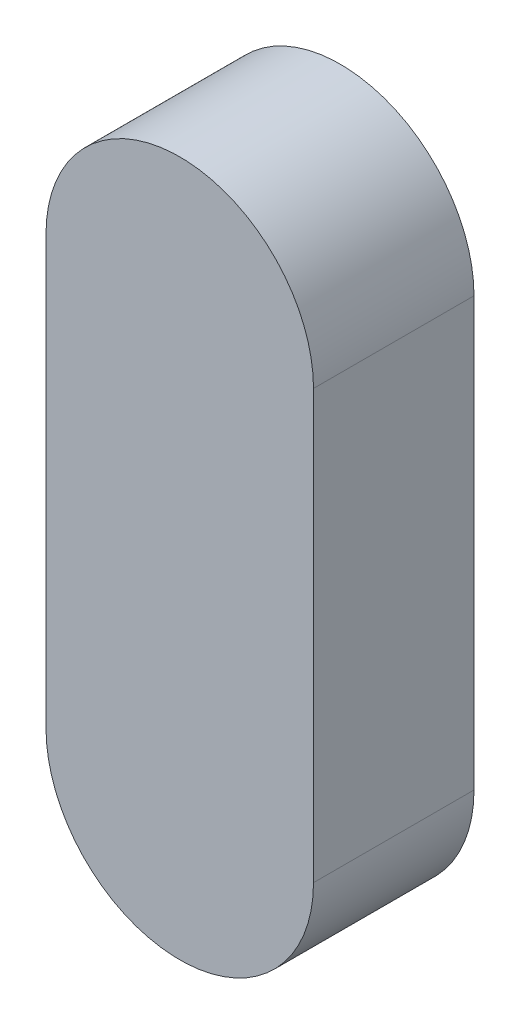
ISO-10303-21;
HEADER;
FILE_DESCRIPTION(('STEP AP214'),'2;1');
FILE_NAME('part.step','',(''),(''),'','','');
FILE_SCHEMA(('AUTOMOTIVE_DESIGN { 1 0 10303 214 1 1 1 1 }'));
ENDSEC;
DATA;
#1=APPLICATION_CONTEXT('core data for automotive mechanical design processes');
#2=APPLICATION_PROTOCOL_DEFINITION('international standard','automotive_design',2000,#1);
#3=PRODUCT_CONTEXT('',#1,'mechanical');
#4=PRODUCT('Part','Part','',(#3));
#5=PRODUCT_RELATED_PRODUCT_CATEGORY('part','',(#4));
#6=PRODUCT_DEFINITION_FORMATION('','',#4);
#7=PRODUCT_DEFINITION_CONTEXT('part definition',#1,'design');
#8=PRODUCT_DEFINITION('design','',#6,#7);
#9=PRODUCT_DEFINITION_SHAPE('','',#8);
#10=(LENGTH_UNIT() NAMED_UNIT(*) SI_UNIT(.MILLI.,.METRE.));
#11=(NAMED_UNIT(*) PLANE_ANGLE_UNIT() SI_UNIT($,.RADIAN.));
#12=(NAMED_UNIT(*) SI_UNIT($,.STERADIAN.) SOLID_ANGLE_UNIT());
#13=UNCERTAINTY_MEASURE_WITH_UNIT(LENGTH_MEASURE(1.E-05),#10,'distance_accuracy_value','');
#14=(GEOMETRIC_REPRESENTATION_CONTEXT(3) GLOBAL_UNCERTAINTY_ASSIGNED_CONTEXT((#13)) GLOBAL_UNIT_ASSIGNED_CONTEXT((#10,
#11,#12)) REPRESENTATION_CONTEXT('',''));
#15=CARTESIAN_POINT('',(0.,0.,0.));
#16=DIRECTION('',(0.,0.,1.));
#17=DIRECTION('',(1.,0.,0.));
#18=AXIS2_PLACEMENT_3D('',#15,#16,#17);
#19=CARTESIAN_POINT('',(0.,0.,3.));
#20=DIRECTION('',(0.,0.,-1.));
#21=DIRECTION('',(-1.,0.,0.));
#22=AXIS2_PLACEMENT_3D('',#19,#20,#21);
#23=CYLINDRICAL_SURFACE('',#22,2.5);
#24=CARTESIAN_POINT('',(0.,0.,0.));
#25=DIRECTION('',(0.,0.,1.));
#26=DIRECTION('',(1.,0.,0.));
#27=AXIS2_PLACEMENT_3D('',#24,#25,#26);
#28=CIRCLE('',#27,2.5);
#29=CARTESIAN_POINT('',(-2.5,0.,0.));
#30=VERTEX_POINT('',#29);
#31=CARTESIAN_POINT('',(2.5,0.,0.));
#32=VERTEX_POINT('',#31);
#33=EDGE_CURVE('E105',#30,#32,#28,.T.);
#34=ORIENTED_EDGE('',*,*,#33,.T.);
#35=DIRECTION('',(0.,0.,-1.));
#36=VECTOR('',#35,1.);
#37=CARTESIAN_POINT('',(2.5,0.,3.));
#38=LINE('',#37,#36);
#39=CARTESIAN_POINT('',(2.5,0.,3.));
#40=VERTEX_POINT('',#39);
#41=EDGE_CURVE('E11',#40,#32,#38,.T.);
#42=ORIENTED_EDGE('',*,*,#41,.F.);
#43=CARTESIAN_POINT('',(0.,0.,3.));
#44=DIRECTION('',(0.,0.,1.));
#45=DIRECTION('',(1.,0.,0.));
#46=AXIS2_PLACEMENT_3D('',#43,#44,#45);
#47=CIRCLE('',#46,2.5);
#48=CARTESIAN_POINT('',(-2.5,0.,3.));
#49=VERTEX_POINT('',#48);
#50=EDGE_CURVE('E89',#49,#40,#47,.T.);
#51=ORIENTED_EDGE('',*,*,#50,.F.);
#52=DIRECTION('',(0.,0.,-1.));
#53=VECTOR('',#52,1.);
#54=CARTESIAN_POINT('',(-2.5,0.,3.));
#55=LINE('',#54,#53);
#56=EDGE_CURVE('E98',#49,#30,#55,.T.);
#57=ORIENTED_EDGE('',*,*,#56,.T.);
#58=EDGE_LOOP('',(#34,#42,#51,#57));
#59=FACE_BOUND('',#58,.T.);
#60=ADVANCED_FACE('F39',(#59),#23,.T.);
#61=CARTESIAN_POINT('',(2.5,0.,3.));
#62=DIRECTION('',(-1.,0.,0.));
#63=DIRECTION('',(0.,-1.,0.));
#64=AXIS2_PLACEMENT_3D('',#61,#62,#63);
#65=PLANE('',#64);
#66=DIRECTION('',(0.,1.,0.));
#67=VECTOR('',#66,1.);
#68=CARTESIAN_POINT('',(2.5,0.,0.));
#69=LINE('',#68,#67);
#70=CARTESIAN_POINT('',(2.5,8.,0.));
#71=VERTEX_POINT('',#70);
#72=EDGE_CURVE('E94',#32,#71,#69,.T.);
#73=ORIENTED_EDGE('',*,*,#72,.T.);
#74=DIRECTION('',(0.,0.,-1.));
#75=VECTOR('',#74,1.);
#76=CARTESIAN_POINT('',(2.5,8.,3.));
#77=LINE('',#76,#75);
#78=CARTESIAN_POINT('',(2.5,8.,3.));
#79=VERTEX_POINT('',#78);
#80=EDGE_CURVE('E50',#79,#71,#77,.T.);
#81=ORIENTED_EDGE('',*,*,#80,.F.);
#82=DIRECTION('',(0.,1.,0.));
#83=VECTOR('',#82,1.);
#84=CARTESIAN_POINT('',(2.5,0.,3.));
#85=LINE('',#84,#83);
#86=EDGE_CURVE('E83',#40,#79,#85,.T.);
#87=ORIENTED_EDGE('',*,*,#86,.F.);
#88=ORIENTED_EDGE('',*,*,#41,.T.);
#89=EDGE_LOOP('',(#73,#81,#87,#88));
#90=FACE_BOUND('',#89,.T.);
#91=ADVANCED_FACE('F91',(#90),#65,.F.);
#92=CARTESIAN_POINT('',(0.,8.,3.));
#93=DIRECTION('',(0.,0.,-1.));
#94=DIRECTION('',(-1.,0.,0.));
#95=AXIS2_PLACEMENT_3D('',#92,#93,#94);
#96=CYLINDRICAL_SURFACE('',#95,2.5);
#97=CARTESIAN_POINT('',(0.,8.,0.));
#98=DIRECTION('',(0.,0.,1.));
#99=DIRECTION('',(1.,0.,0.));
#100=AXIS2_PLACEMENT_3D('',#97,#98,#99);
#101=CIRCLE('',#100,2.5);
#102=CARTESIAN_POINT('',(-2.5,8.,0.));
#103=VERTEX_POINT('',#102);
#104=EDGE_CURVE('E75',#71,#103,#101,.T.);
#105=ORIENTED_EDGE('',*,*,#104,.T.);
#106=DIRECTION('',(0.,0.,-1.));
#107=VECTOR('',#106,1.);
#108=CARTESIAN_POINT('',(-2.5,8.,3.));
#109=LINE('',#108,#107);
#110=CARTESIAN_POINT('',(-2.5,8.,3.));
#111=VERTEX_POINT('',#110);
#112=EDGE_CURVE('E92',#111,#103,#109,.T.);
#113=ORIENTED_EDGE('',*,*,#112,.F.);
#114=CARTESIAN_POINT('',(0.,8.,3.));
#115=DIRECTION('',(0.,0.,1.));
#116=DIRECTION('',(1.,0.,0.));
#117=AXIS2_PLACEMENT_3D('',#114,#115,#116);
#118=CIRCLE('',#117,2.5);
#119=EDGE_CURVE('E86',#79,#111,#118,.T.);
#120=ORIENTED_EDGE('',*,*,#119,.F.);
#121=ORIENTED_EDGE('',*,*,#80,.T.);
#122=EDGE_LOOP('',(#105,#113,#120,#121));
#123=FACE_BOUND('',#122,.T.);
#124=ADVANCED_FACE('F96',(#123),#96,.T.);
#125=CARTESIAN_POINT('',(-2.5,0.,3.));
#126=DIRECTION('',(1.,0.,0.));
#127=DIRECTION('',(0.,1.,0.));
#128=AXIS2_PLACEMENT_3D('',#125,#126,#127);
#129=PLANE('',#128);
#130=DIRECTION('',(0.,-1.,0.));
#131=VECTOR('',#130,1.);
#132=CARTESIAN_POINT('',(-2.5,0.,0.));
#133=LINE('',#132,#131);
#134=EDGE_CURVE('E79',#103,#30,#133,.T.);
#135=ORIENTED_EDGE('',*,*,#134,.T.);
#136=ORIENTED_EDGE('',*,*,#56,.F.);
#137=DIRECTION('',(0.,-1.,0.));
#138=VECTOR('',#137,1.);
#139=CARTESIAN_POINT('',(-2.5,0.,3.));
#140=LINE('',#139,#138);
#141=EDGE_CURVE('E54',#111,#49,#140,.T.);
#142=ORIENTED_EDGE('',*,*,#141,.F.);
#143=ORIENTED_EDGE('',*,*,#112,.T.);
#144=EDGE_LOOP('',(#135,#136,#142,#143));
#145=FACE_BOUND('',#144,.T.);
#146=ADVANCED_FACE('F108',(#145),#129,.F.);
#147=CARTESIAN_POINT('',(0.,0.,3.));
#148=DIRECTION('',(0.,0.,1.));
#149=DIRECTION('',(1.,0.,0.));
#150=AXIS2_PLACEMENT_3D('',#147,#148,#149);
#151=PLANE('',#150);
#152=ORIENTED_EDGE('',*,*,#50,.T.);
#153=ORIENTED_EDGE('',*,*,#86,.T.);
#154=ORIENTED_EDGE('',*,*,#119,.T.);
#155=ORIENTED_EDGE('',*,*,#141,.T.);
#156=EDGE_LOOP('',(#152,#153,#154,#155));
#157=FACE_BOUND('',#156,.T.);
#158=ADVANCED_FACE('F88',(#157),#151,.T.);
#159=CARTESIAN_POINT('',(0.,0.,0.));
#160=DIRECTION('',(0.,0.,1.));
#161=DIRECTION('',(1.,0.,0.));
#162=AXIS2_PLACEMENT_3D('',#159,#160,#161);
#163=PLANE('',#162);
#164=ORIENTED_EDGE('',*,*,#33,.F.);
#165=ORIENTED_EDGE('',*,*,#134,.F.);
#166=ORIENTED_EDGE('',*,*,#104,.F.);
#167=ORIENTED_EDGE('',*,*,#72,.F.);
#168=EDGE_LOOP('',(#164,#165,#166,#167));
#169=FACE_BOUND('',#168,.T.);
#170=ADVANCED_FACE('F115',(#169),#163,.F.);
#171=CLOSED_SHELL('',(#60,#91,#124,#146,#158,#170));
#172=MANIFOLD_SOLID_BREP('B2',#171);
#173=ADVANCED_BREP_SHAPE_REPRESENTATION('',(#18,#172),#14);
#174=SHAPE_DEFINITION_REPRESENTATION(#9,#173);
ENDSEC;
END-ISO-10303-21;
